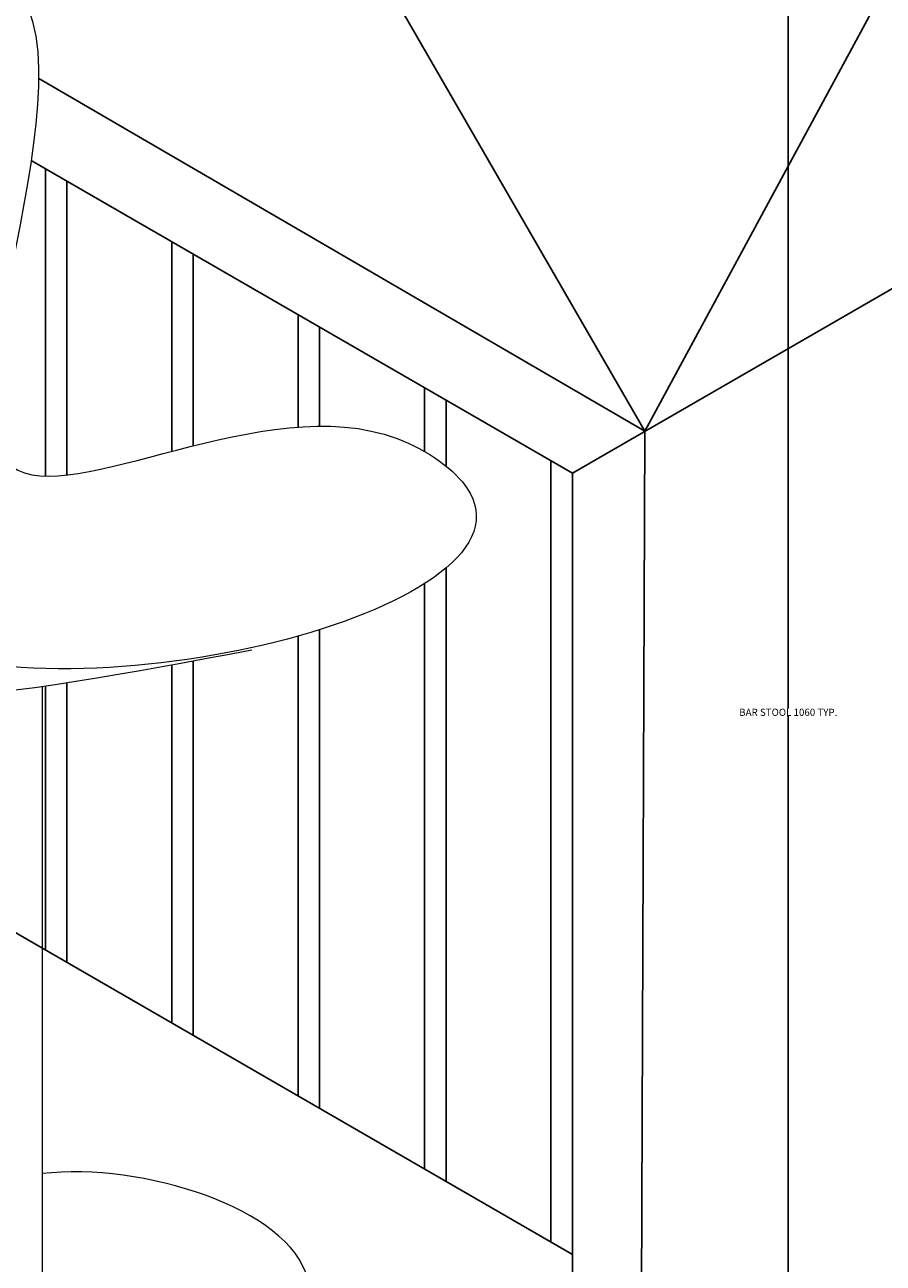
# Model space of a CAD drawing. Units: metres. Extents: x -2391 to 4922, y -635 to 4845.
# Tile 8 of 37: x -871 to -271, y 53 to 919. Entities that reach past the tile are written whole.
import ezdxf

# ---------------------------------------------------------------- set-up
doc = ezdxf.new("R2010")
doc.units = ezdxf.units.M
doc.header["$MEASUREMENT"] = 0
for name, color, linetype, lineweight in [('A-ANNO-DIMS', 2, 'Continuous', 18), ('A-FLOR-FIXT', 3, 'Continuous', 25), ('A-FURN', 8, 'Continuous', 18)]:
    doc.layers.add(name, color=color, linetype=linetype, lineweight=lineweight)
doc.styles.get("Standard").update_dxf_attribs({"font": 'arial.ttf'})
doc.dimstyles.get("Standard").update_dxf_attribs({"dimtxt": 5, "dimasz": 4, "dimexe": 0.18, "dimexo": 0.0625, "dimgap": 0.09, "dimtad": 0, "dimtih": 1, "dimtoh": 1, "dimdec": 0, "dimzin": 0, "dimdsep": 46, "dimtxsty": 'Standard', "dimcen": 0.09, "dimadec": 0, "dimazin": 0, "dimtfac": 1, "dimtdec": 0, "dimtofl": 0, "dimtmove": 0, "dimatfit": 3, "dimfxl": 1, "dimtolj": 1, "dimtzin": 0, "dimarcsym": 0})

# ---------------------------------------------------------------- blocks, each defined once
blk = doc.blocks.new('STOOL-BAR')
blk.add_line((227.15, 541.57), (227.15, 114.21))
for points, knots in [([(47.24, 931.27), (26.82, 772.78), (-15.55, 443.76), (639.86, 614.21), (403.75, 766.18), (59.87, 548.32), (308.37, 1061.03), (87.86, 1049.28), (63.7, 979.1), (47.24, 931.27)], [0, 0, 0, 0, 373.373325, 775.091582, 839.205201, 1103.589215, 1452.822506, 1516.235646, 1651.960559, 1651.960559, 1651.960559, 1651.960559]), ([(82.71, 605.1), (79.37, 599.07), (25.39, 501.43), (205.15, 535.32), (373.81, 567.12)], [0, 0, 0, 0, 19.816883, 320.720948, 320.720948, 320.720948, 320.720948]), ([(193.66, 199.14), (106.89, 200.34), (-113.88, 203.37), (215.44, -95.9), (508.37, 143.53), (296.52, 208.79), (227.15, 200.77)], [0, 0, 0, 0, 131.596892, 334.838301, 476.929251, 613.088937, 613.088937, 613.088937, 613.088937])]:
    blk.add_open_spline(points, degree=3, knots=knots)
blk = doc.blocks.new('*D6')
at = {"layer": 'A-ANNO-DIMS', "color": 0, "lineweight": -2, "transparency": 16777216}
for p, q in [((-496.54, 968.1), (-337.38, 968.1)), ((-337.56, 964.1), (-337.56, 440.64)), ((-337.56, -88.18), (-337.56, 435.28)), ((-496.54, -92.18), (-337.38, -92.18))]:
    blk.add_line(p, q, dxfattribs=at)
at = {"layer": 'A-ANNO-DIMS', "color": 0, "transparency": 16777216}
for points in [[(-338.23, 964.1), (-336.89, 964.1), (-337.56, 968.1)], [(-338.23, -88.18), (-336.89, -88.18), (-337.56, -92.18)]]:
    blk.add_solid(points, dxfattribs=at)
at = {"layer": 'Defpoints', "color": 0, "transparency": 16777216}
for p in [(-496.6, 968.1), (-337.56, 968.1), (-496.6, -92.18)]:
    blk.add_point(p, dxfattribs=at)
at = {"layer": 'A-ANNO-DIMS', "color": 0, "transparency": 16777216, "insert": (-337.56, 437.96), "char_height": 5, "attachment_point": 5}
blk.add_mtext('\\A1;BAR STOOL 1060 TYP.', dxfattribs=at)
blk = doc.blocks.new('*D8')
at = {"layer": 'A-ANNO-DIMS', "color": 0, "lineweight": -2, "transparency": 16777216}
for p, q in [((-2047.33, 3005.21), (-2047.33, -631.4)), ((4577.76, 2350.21), (4577.76, -631.4)), ((-2043.33, -631.22), (1257.62, -631.22)), ((4573.76, -631.22), (1272.8, -631.22))]:
    blk.add_line(p, q, dxfattribs=at)
at = {"layer": 'A-ANNO-DIMS', "color": 0, "transparency": 16777216}
for points in [[(-2043.33, -630.56), (-2043.33, -631.89), (-2047.33, -631.22)], [(4573.76, -630.56), (4573.76, -631.89), (4577.76, -631.22)]]:
    blk.add_solid(points, dxfattribs=at)
at = {"layer": 'Defpoints', "color": 0, "transparency": 16777216}
for p in [(-2047.33, 3005.28), (4577.76, 2350.28), (4577.76, -631.22)]:
    blk.add_point(p, dxfattribs=at)
at = {"layer": 'A-ANNO-DIMS', "color": 0, "transparency": 16777216, "insert": (1265.21, -631.22), "char_height": 5, "attachment_point": 5}
blk.add_mtext('\\A1;6625', dxfattribs=at)
blk = doc.blocks.new('*D10')
at = {"layer": 'A-ANNO-DIMS', "color": 0, "lineweight": -2, "transparency": 16777216}
for p, q in [((550.68, 4505.28), (-2384.01, 4505.28)), ((-2383.83, 4501.28), (-2383.83, 2107.92)), ((-2383.83, -290.72), (-2383.83, 2102.63)), ((-488.55, -294.72), (-2384.01, -294.72))]:
    blk.add_line(p, q, dxfattribs=at)
at = {"layer": 'A-ANNO-DIMS', "color": 0, "transparency": 16777216}
for points in [[(-2384.5, 4501.28), (-2383.17, 4501.28), (-2383.83, 4505.28)], [(-2384.5, -290.72), (-2383.17, -290.72), (-2383.83, -294.72)]]:
    blk.add_solid(points, dxfattribs=at)
at = {"layer": 'Defpoints', "color": 0, "transparency": 16777216}
for p in [(-2383.83, 4505.28), (550.74, 4505.28), (-488.49, -294.72)]:
    blk.add_point(p, dxfattribs=at)
at = {"layer": 'A-ANNO-DIMS', "color": 0, "transparency": 16777216, "insert": (-2383.83, 2105.28), "char_height": 5, "attachment_point": 5}
blk.add_mtext('\\A1;4800', dxfattribs=at)
blk = doc.blocks.new('*D46')
at = {"layer": 'A-ANNO-DIMS', "color": 0, "lineweight": -2, "transparency": 16777216}
for p, q in [((-2047.3, 1505.33), (-1887.13, 1801.4)), ((-1883.7, 1799.34), (-1087.36, 1368.5)), ((-281.24, 932.38), (-1077.58, 1363.21)), ((-437.81, 634.57), (-277.64, 930.64))]:
    blk.add_line(p, q, dxfattribs=at)
at = {"layer": 'A-ANNO-DIMS', "color": 0, "transparency": 16777216}
for points in [[(-1883.38, 1799.92), (-1884.01, 1798.75), (-1887.21, 1801.24)], [(-280.92, 932.97), (-281.56, 931.8), (-277.72, 930.48)]]:
    blk.add_solid(points, dxfattribs=at)
at = {"layer": 'Defpoints', "color": 0, "transparency": 16777216}
for p in [(-2047.33, 1505.28), (-277.72, 930.48), (-437.84, 634.52)]:
    blk.add_point(p, dxfattribs=at)
at = {"layer": 'A-ANNO-DIMS', "color": 0, "transparency": 16777216, "insert": (-1082.47, 1365.86), "char_height": 5, "attachment_point": 5}
blk.add_mtext('\\A1;1830', dxfattribs=at)
blk = doc.blocks.new('*D47')
at = {"layer": 'A-ANNO-DIMS', "color": 0, "lineweight": -2, "transparency": 16777216}
for p, q in [((31.1, 905.33), (-137.21, 1196.85)), ((-140.59, 1194.69), (-367.03, 1063.96)), ((-602.63, 927.94), (-376.18, 1058.67)), ((-437.87, 634.57), (-606.18, 926.09))]:
    blk.add_line(p, q, dxfattribs=at)
at = {"layer": 'A-ANNO-DIMS', "color": 0, "transparency": 16777216}
for points in [[(-140.92, 1195.27), (-140.25, 1194.12), (-137.12, 1196.69)], [(-602.96, 928.51), (-602.29, 927.36), (-606.09, 925.94)]]:
    blk.add_solid(points, dxfattribs=at)
at = {"layer": 'Defpoints', "color": 0, "transparency": 16777216}
for p in [(-137.12, 1196.69), (31.13, 905.28), (-437.84, 634.52)]:
    blk.add_point(p, dxfattribs=at)
at = {"layer": 'A-ANNO-DIMS', "color": 0, "transparency": 16777216, "insert": (-371.61, 1061.31), "char_height": 5, "attachment_point": 5}
blk.add_mtext('\\A1;541.5', dxfattribs=at)

msp = doc.modelspace()

# ---------------------------------------------------------------- linework, layer by layer
at = {"layer": 'A-FLOR-FIXT'}
for p, q in [((31.1266, 905.2763), (-488.4886, 605.2763)), ((-861.7634, 881.3083), (-437.841, 634.5176)), ((-488.4886, 605.2763), (-866.9799, 823.7983)), ((-857.1025, 818.0956), (-857.1025, 603.1613)), ((-842.0944, 809.4307), (-842.0944, 603.9009)), ((-1741.1171, 782.0708), (-488.4886, 58.8654)), ((-768.7011, 767.057), (-768.7011, 620.4789)), ((-753.693, 758.3921), (-753.693, 624.3158)), ((-680.2996, 716.0184), (-680.2996, 637.45)), ((-665.2915, 707.3535), (-665.2915, 638.0851)), ((-591.8981, 664.9798), (-591.8981, 620.3679)), ((-576.8901, 656.3149), (-576.8901, 610.1847)), ((-437.841, 634.5176), (-441.31, -267.4852)), ((-503.4967, 613.9412), (-503.4967, 67.5303)), ((-488.4886, 605.2763), (-488.4886, -294.7237)), ((-488.4886, 605.2763), (-488.4886, 58.8654)), ((-576.8901, 538.8867), (-576.8901, 109.904)), ((-591.8981, 527.9404), (-591.8981, 118.5689)), ((-665.2915, 495.7531), (-665.2915, 160.9426)), ((-680.2996, 491.29), (-680.2996, 169.6075)), ((-768.7011, 471.2062), (-768.7011, 220.6462)), ((-753.693, 473.9709), (-753.693, 211.9812)), ((-857.1025, 456.4326), (-857.1025, 271.6848)), ((-842.0944, 458.6686), (-842.0944, 263.0198))]:
    msp.add_line(p, q, dxfattribs=at)

# ---------------------------------------------------------------- block references
at = {"layer": 'A-FURN'}
msp.add_blockref('STOOL-BAR', (-1086.3941, -85.4426), dxfattribs=at)

# ---------------------------------------------------------------- dimensions: what is measured, and where the dimension line sits
at = {"layer": 'A-ANNO-DIMS'}
for base, p1, p2, angle, override, picture, middle in [((-2383.8343, 4505.2763), (-488.4886, -294.7237), (550.7419, 4505.2763), 90, {"dimdec": 0, "dimlfac": 1, "dimrnd": 0, "dimzin": 0, "dimdsep": 46, "dimlunit": 2}, '*D10', (-2383.8343, 2105.2763)), ((-277.7211, 930.4802), (-2047.3343, 1505.2763), (-437.841, 634.5176), 331.5859855, {"dimdec": 0, "dimlfac": 1, "dimrnd": 0, "dimzin": 0, "dimdsep": 46, "dimlunit": 2}, '*D46', (-1082.4677, 1365.8595)), ((-137.1234, 1196.6938), (-437.841, 634.5176), (31.1266, 905.2763), 30, {"dimdec": 1, "dimlfac": 1, "dimrnd": 0, "dimzin": 0, "dimdsep": 46, "dimlunit": 2}, '*D47', (-371.6072, 1061.3145))]:
    dim = msp.add_linear_dim(base=base, p1=p1, p2=p2, angle=angle, dimstyle='Standard', override=override, dxfattribs=at)
    dim.commit()
    dim.dimension.update_dxf_attribs({"geometry": picture, "text_midpoint": middle})
dim = msp.add_linear_dim(base=(4577.76, -631.2237), p1=(-2047.3343, 3005.2763), p2=(4577.76, 2350.2763), dimstyle='Standard', override={"dimdec": 0, "dimlfac": 1, "dimrnd": 0, "dimzin": 0, "dimdsep": 46, "dimlunit": 2}, dxfattribs=at)
dim.commit()
dim.dimension.update_dxf_attribs({"geometry": '*D8', "text_midpoint": (1265.2128, -631.2237)})
dim = msp.add_linear_dim(base=(-337.5616, 968.1038), p1=(-496.6042, -92.1799), p2=(-496.6042, 968.1038), angle=90, text='BAR STOOL <> TYP.', dimstyle='Standard', override={"dimdec": 0, "dimrnd": 0, "dimzin": 0, "dimlunit": 2}, dxfattribs=at)
dim.commit()
dim.dimension.update_dxf_attribs({"geometry": '*D6', "text_midpoint": (-337.5616, 437.9619)})

doc.saveas('drawing.dxf')
